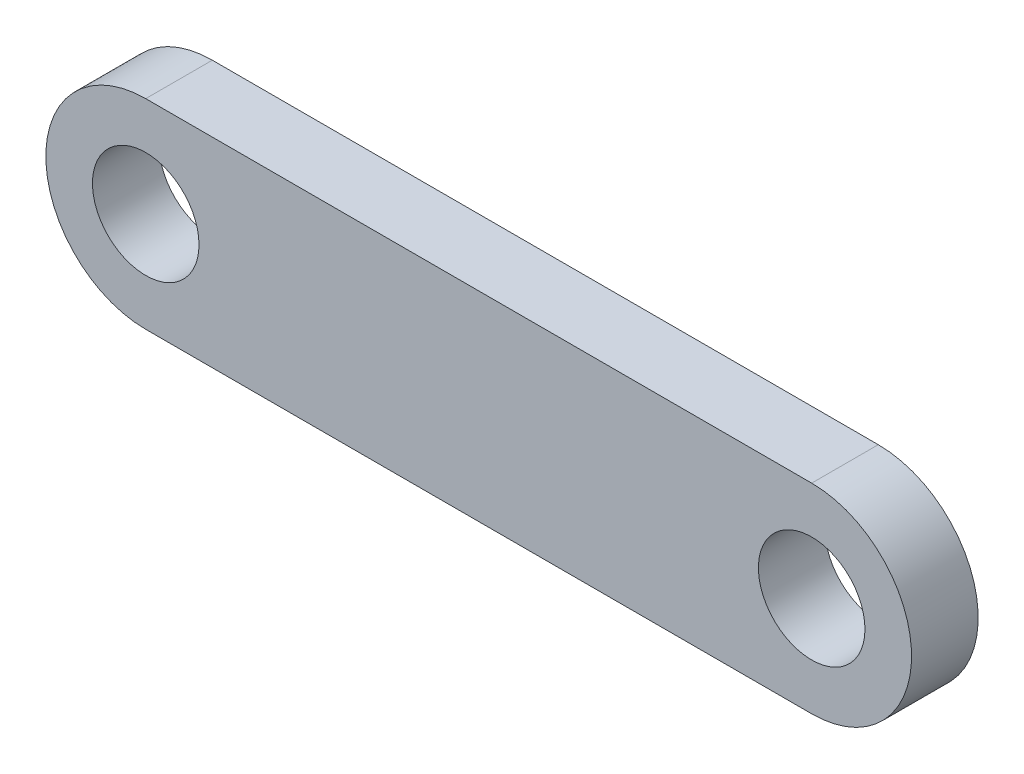
from build123d import *

# Parameters (mm, degrees)
LINK_PLATE_PROFILE_SKETCH_R          = 4
LINK_PLATE_5MM_WITH_HOLES_2X_8_DEPTH = 2.5


with BuildPart() as part:
    # Link Plate Profile Sketch → Link Plate 5mm with Holes 2xØ8 (new, symmetric)
    with BuildSketch(Plane.XY):
        with BuildLine():
            Line((25, -7.5), (-25, -7.5))
            ThreePointArc((-25, -7.5), (-32.5, 0), (-25, 7.5))
            Line((-25, 7.5), (25, 7.5))
            ThreePointArc((25, 7.5), (32.5, 0), (25, -7.5))
        make_face()
        with Locations((-25, 0)):
            Circle(LINK_PLATE_PROFILE_SKETCH_R, mode=Mode.SUBTRACT)
        with Locations((25, 0)):
            Circle(LINK_PLATE_PROFILE_SKETCH_R, mode=Mode.SUBTRACT)
    extrude(amount=LINK_PLATE_5MM_WITH_HOLES_2X_8_DEPTH, both=True)


solid = part.part
